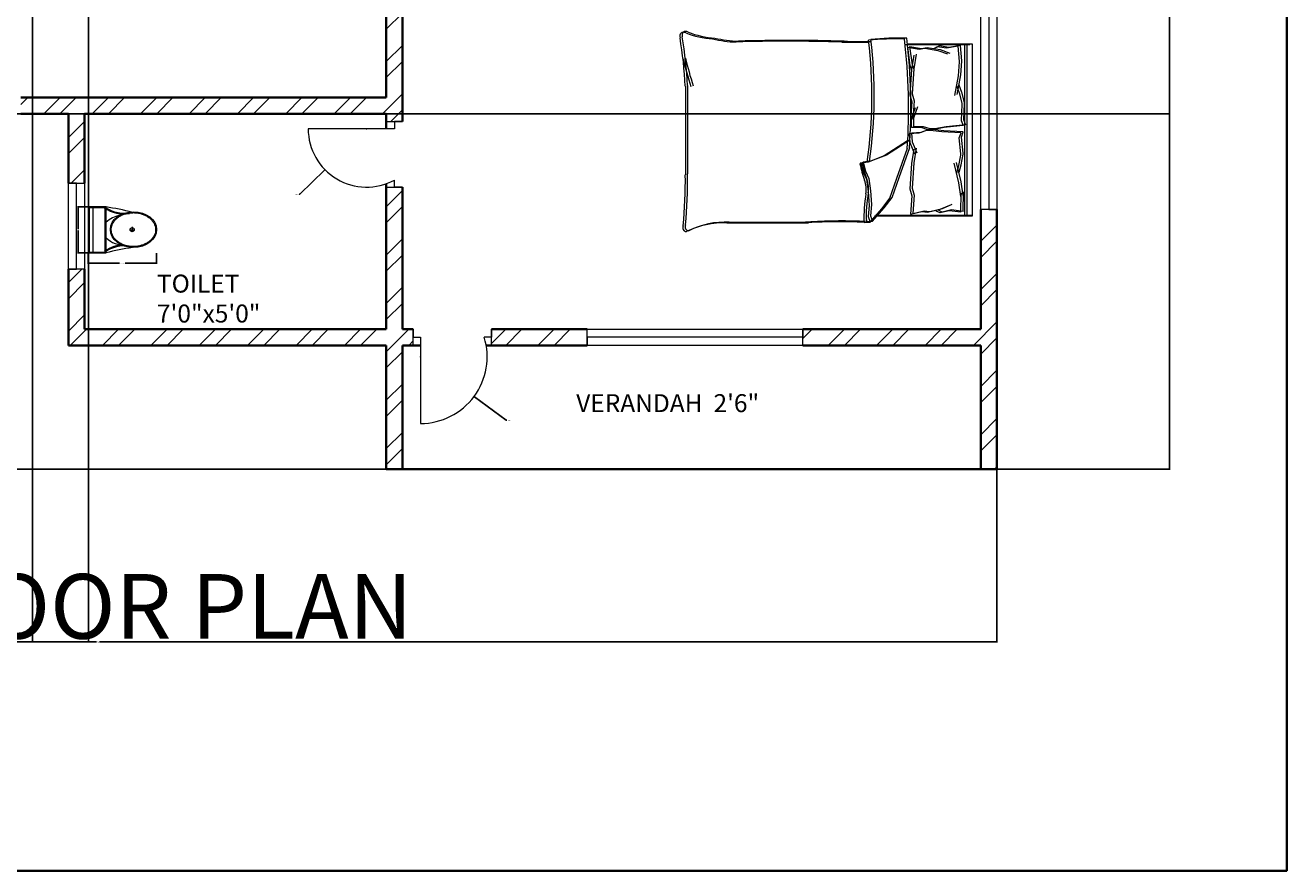
# Model space of a CAD drawing. Units: inches. Extents: x 2008 to 2657, y 1077 to 2165.
# Tile 5 of 16: x 2306 to 2657, y 1077 to 1312. Entities that reach past the tile are written whole.
import ezdxf

# ---------------------------------------------------------------- set-up
doc = ezdxf.new("R2010")
doc.units = ezdxf.units.IN
for name, color, linetype, lineweight in [('A-ANNO-DIMS', 2, 'Continuous', 18), ('A-ANNO-TITL', 7, 'Continuous', 35), ('A-ANNO-TTLB', 7, 'Continuous', 35), ('A-AREA-IDEN', 4, 'Continuous', 18), ('A-DOOR', 11, 'Continuous', 18), ('A-FLOR-FIXT', 8, 'Continuous', 18), ('A-FURN', 8, 'Continuous', 13), ('A-GLAZ', 191, 'Continuous', 18), ('A-WALL', 7, 'Continuous', 35)]:
    doc.layers.add(name, color=color, linetype=linetype, lineweight=lineweight)
doc.layers.add('A-WALL-PATT', color=30, linetype='Continuous', lineweight=13, true_color=0xf8991e)
doc.styles.get("Standard").update_dxf_attribs({"font": 'arial.ttf'})
doc.dimstyles.get("Standard").update_dxf_attribs({"dimtxt": 0.18, "dimasz": 0.18, "dimexe": 0.18, "dimexo": 0.0625, "dimgap": 0.09, "dimtad": 0, "dimtih": 1, "dimtoh": 1, "dimdec": 4, "dimzin": 0, "dimdsep": 46, "dimtxsty": 'Standard', "dimcen": 0.09, "dimadec": 0, "dimazin": 0, "dimtfac": 1, "dimtdec": 4, "dimtofl": 0, "dimtmove": 0, "dimatfit": 3, "dimfxl": 1, "dimtolj": 1, "dimtzin": 0, "dimarcsym": 0})

# ---------------------------------------------------------------- blocks, each defined once
blk = doc.blocks.new('A$C31115884')
for p, q in [((283, 498), (223, 498)), ((258, 466), (258, 523)), ((0, 200), (0, 0)), ((520, 200), (0, 200)), ((10, 190), (10, 10)), ((510, 190), (10, 190)), ((510, 10), (510, 190)), ((520, 0), (520, 200)), ((510, 54), (0, 54)), ((10, 10), (510, 10)), ((0, 0), (520, 0))]:
    blk.add_line(p, q)
blk.add_circle((256, 496), 23.6)
for centre, radius, start, end in [((2778, -205), 2807, 165.4549, 171.7133), ((-295, 403), 365, 324.2091, 9.3499), ((-295, 403), 375, 324.2091, 9.3499), ((806, 403), 365, 170.6501, 215.7909), ((3237, 905), 2807, 188.2867, 194.5451), ((384, 406), 293, 190.2774, 224.1564), ((139, 406), 293, 315.8436, 2.6563), ((806, 403), 375, 179.2036, 215.7909)]:
    blk.add_arc(centre, radius, start, end)
blk.add_ellipse((256, 510), major_axis=(0, -261), ratio=0.772727)
blk.add_open_spline([(256, 259), (263, 259), (270, 260), (288, 262), (299, 265), (320, 273), (330, 278), (350, 291), (360, 299), (378, 316), (386, 326), (402, 347), (409, 358), (421, 383), (427, 395), (436, 422), (440, 436), (445, 465), (447, 480), (448, 509), (448, 524), (445, 553), (443, 568), (436, 596), (432, 610), (422, 636), (416, 649), (402, 672), (395, 683), (379, 703), (370, 712), (351, 728), (341, 735), (321, 746), (310, 751), (289, 757), (278, 759), (256, 761), (245, 761), (223, 757), (212, 754), (191, 746), (181, 741), (161, 728), (151, 720), (133, 703), (125, 693), (110, 672), (103, 660), (90, 636), (85, 623), (76, 596), (72, 582), (67, 553), (66, 538), (64, 509), (65, 494), (68, 465), (70, 450), (77, 422), (81, 408), (91, 382), (97, 370), (111, 346), (118, 335), (135, 316), (144, 307), (162, 291), (172, 284), (193, 273), (203, 269), (225, 262), (236, 260), (250, 259), (253, 259), (256, 259)], degree=3, knots=[0, 0, 0, 0, 0.110105, 0.110105, 0.285049, 0.285049, 0.459994, 0.459994, 0.634938, 0.634938, 0.809882, 0.809882, 0.984827, 0.984827, 1.159771, 1.159771, 1.334715, 1.334715, 1.50966, 1.50966, 1.684604, 1.684604, 1.859549, 1.859549, 2.034493, 2.034493, 2.209437, 2.209437, 2.384382, 2.384382, 2.559326, 2.559326, 2.73427, 2.73427, 2.909215, 2.909215, 3.084159, 3.084159, 3.259103, 3.259103, 3.434048, 3.434048, 3.608992, 3.608992, 3.783936, 3.783936, 3.958881, 3.958881, 4.133825, 4.133825, 4.30877, 4.30877, 4.483714, 4.483714, 4.658658, 4.658658, 4.833603, 4.833603, 5.008547, 5.008547, 5.183491, 5.183491, 5.358436, 5.358436, 5.53338, 5.53338, 5.708324, 5.708324, 5.883269, 5.883269, 6.058213, 6.058213, 6.233158, 6.233158, 6.283185, 6.283185, 6.283185, 6.283185])
blk = doc.blocks.new('BED-DOUBLE')
for p, q in [((27.75, 52.87), (24.5, 49.16)), ((27.75, 52.87), (24.5, 49.16)), ((28.39, 53.1), (25.14, 49.39)), ((28.39, 53.1), (25.14, 49.39)), ((29.49, 52.95), (27.75, 52.87, 3.87)), ((29.49, 52.95), (27.75, 52.87, 3.87)), ((28.37, 51.33), (27.75, 52.87)), ((28.37, 51.33), (27.75, 52.87)), ((30.13, 53.18), (28.39, 53.1, 3.87)), ((30.13, 53.18), (28.39, 53.1, 3.87)), ((29, 51.56), (28.39, 53.1)), ((29, 51.56), (28.39, 53.1)), ((0, 51.49), (0.64, 51.49)), ((0, 3.48), (0, 51.49)), ((0, 51.27), (26.61, 51.27)), ((0, 51.27), (26.61, 51.27)), ((0.64, 51.49), (27.25, 51.49)), ((0.64, 51.49), (27.25, 51.49)), ((1.53, 3.48), (1.53, 51.27)), ((1.53, 3.48), (1.53, 51.27)), ((2.17, 3.7), (2.17, 51.49)), ((2.17, 3.7), (2.17, 51.49)), ((2.56, 50.11), (2.46, 44.71)), ((2.56, 50.11), (2.46, 44.71)), ((2.56, 50.11), (5.77, 49.73)), ((2.56, 50.11), (5.77, 49.73)), ((3.2, 50.34), (3.1, 44.94)), ((3.2, 50.34), (3.1, 44.94)), ((3.2, 50.34), (6.41, 49.96)), ((3.2, 50.34), (6.41, 49.96)), ((8.26, 49.31), (5.58, 48.13)), ((8.26, 49.31), (5.58, 48.13)), ((5.77, 49.73), (8.34, 50.33)), ((5.77, 49.73), (8.34, 50.33)), ((8.9, 49.54), (6.22, 48.36)), ((8.9, 49.54), (6.22, 48.36)), ((6.41, 49.96), (8.98, 50.56)), ((6.41, 49.96), (8.98, 50.56)), ((11.83, 50.11), (8.26, 49.31)), ((11.83, 50.11), (8.26, 49.31)), ((8.34, 50.33), (9.38, 49.82)), ((8.34, 50.33), (9.38, 49.81)), ((12.47, 50.34), (8.9, 49.54)), ((12.47, 50.34), (8.9, 49.54)), ((8.98, 50.56), (10.02, 50.04)), ((8.98, 50.56), (10.02, 50.04)), ((13.43, 49.92), (11.83, 50.11)), ((13.43, 49.92), (11.83, 50.11)), ((14.07, 50.15), (12.47, 50.34)), ((14.07, 50.15), (12.47, 50.34)), ((16.57, 50.7), (13.43, 49.92)), ((16.57, 50.7), (13.43, 49.92)), ((17.21, 50.93), (14.07, 50.15)), ((17.21, 50.93), (14.07, 50.15)), ((16.17, 45.57), (16.57, 50.7)), ((16.17, 45.57), (16.57, 50.7)), ((16.81, 45.8), (17.21, 50.93)), ((16.81, 45.8), (17.21, 50.93)), ((25.14, 49.39), (22.97, 46.45)), ((25.14, 49.39), (22.97, 46.45)), ((28.06, 48.23), (28.37, 51.33)), ((28.06, 48.23), (28.37, 51.33)), ((28.7, 48.46), (29, 51.56)), ((28.7, 48.46), (29, 51.56)), ((2.46, 44.71), (2.54, 45.71)), ((2.46, 44.71), (2.54, 45.71)), ((2.54, 45.71), (3.07, 41.91)), ((2.54, 45.71), (3.07, 41.91)), ((3.1, 44.94), (3.18, 45.94)), ((3.1, 44.94), (3.18, 45.94)), ((3.18, 45.94), (3.71, 42.14)), ((3.18, 45.94), (3.71, 42.14)), ((17.37, 43.84), (16.81, 45.8)), ((17.37, 43.83), (16.81, 45.8)), ((22.33, 46.22), (20.32, 40.64)), ((22.33, 46.22), (20.32, 40.64)), ((22.97, 46.45), (20.96, 40.87)), ((22.97, 46.45), (20.96, 40.87)), ((24.5, 49.16), (22.33, 46.22)), ((24.5, 49.16), (22.33, 46.22)), ((28.37, 44.36), (28.06, 48.23)), ((28.37, 44.36), (28.06, 48.23)), ((29, 44.59), (28.7, 48.46)), ((29, 44.59), (28.7, 48.46)), ((16.73, 43.61), (16.17, 45.57)), ((16.73, 43.61), (16.17, 45.57)), ((16.3, 36.6), (16.73, 43.61)), ((16.3, 36.6), (16.73, 43.61)), ((16.93, 36.83), (17.37, 43.84)), ((16.93, 36.82), (17.37, 43.83)), ((28.83, 40.95), (28.37, 44.36)), ((28.83, 40.95), (28.37, 44.36)), ((29.47, 41.18), (29, 44.59)), ((29.47, 41.18), (29, 44.59)), ((3.07, 41.91), (4.42, 36.5)), ((3.07, 41.91), (4.42, 36.5)), ((3.67, 39.2), (3.08, 37.14)), ((3.67, 39.2), (3.08, 37.14)), ((3.71, 42.14), (5.06, 36.72)), ((3.71, 42.14), (5.06, 36.72)), ((4.31, 39.43), (3.72, 37.36)), ((4.31, 39.43), (3.72, 37.36)), ((20.32, 40.64), (17.38, 32.31)), ((20.32, 40.64), (17.38, 32.31)), ((20.96, 40.87), (18.02, 32.54)), ((20.96, 40.87), (18.02, 32.53)), ((29.76, 38.94), (28.83, 40.95)), ((29.76, 38.94), (28.83, 40.95)), ((30.4, 39.17), (29.47, 41.18)), ((30.4, 39.17), (29.47, 41.18)), ((30.38, 36.46), (29.76, 38.94)), ((30.38, 36.46), (29.76, 38.94)), ((31.02, 36.69), (30.4, 39.17)), ((31.02, 36.69), (30.4, 39.17)), ((79.25, 15.06), (79.25, 39.68)), ((79.25, 15.06), (79.25, 39.68)), ((79.88, 15.29), (79.88, 39.91)), ((79.88, 15.29), (79.88, 39.91)), ((3.08, 37.14), (2.54, 34.21)), ((3.08, 37.14), (2.54, 34.2)), ((3.72, 37.36), (3.18, 34.43)), ((3.72, 37.36), (3.18, 34.43)), ((15.63, 32.56), (16.3, 36.6)), ((15.63, 32.56), (16.3, 36.6)), ((16.27, 32.79), (16.93, 36.83)), ((16.27, 32.79), (16.93, 36.82)), ((23.88, 34.45), (28.37, 36.15)), ((23.88, 34.45), (28.37, 36.15)), ((24.52, 34.68), (29, 36.38)), ((24.52, 34.68), (29, 36.38)), ((28.37, 36.15), (30.38, 36.46)), ((28.37, 36.15), (30.38, 36.46)), ((29, 36.38), (31.02, 36.69)), ((29, 36.38), (31.02, 36.69)), ((2.54, 34.21), (2.56, 33.88)), ((2.54, 34.2), (2.56, 33.88)), ((2.56, 33.88), (2.98, 29.46)), ((2.56, 33.88), (2.98, 29.46)), ((3.18, 34.43), (3.2, 34.11)), ((3.18, 34.43), (3.2, 34.11)), ((3.2, 34.11), (3.62, 29.68)), ((3.2, 34.11), (3.62, 29.68)), ((16.74, 30.75), (15.45, 33.82)), ((16.74, 30.75), (15.45, 33.82)), ((17.38, 30.98), (16.09, 34.05)), ((17.38, 30.98), (16.09, 34.05)), ((17.38, 30.26), (23.88, 34.45)), ((17.38, 30.26), (23.88, 34.45)), ((18.02, 30.49), (24.52, 34.68)), ((18.02, 30.49), (24.52, 34.68)), ((2.98, 29.46), (2.49, 27.98)), ((2.98, 29.46), (2.49, 27.98)), ((3.62, 29.68), (3.13, 28.21)), ((3.62, 29.68), (3.13, 28.21)), ((3.13, 28.21), (8.51, 27.96)), ((3.13, 28.21), (8.51, 27.96)), ((12.38, 27.44), (14.22, 28.13)), ((12.38, 27.44), (14.22, 28.13)), ((13.02, 27.66), (14.86, 28.36)), ((13.02, 27.66), (14.86, 28.36)), ((14.22, 28.13), (16.89, 28.3)), ((14.22, 28.13), (16.89, 28.3)), ((14.86, 28.36), (17.53, 28.53)), ((14.86, 28.36), (17.53, 28.53)), ((16.89, 28.3), (16.74, 30.75)), ((16.89, 28.3), (16.74, 30.75)), ((17.53, 28.53), (17.38, 30.98)), ((17.53, 28.53), (17.38, 30.98)), ((1.87, 25.98), (7.22, 26.56)), ((1.87, 25.98), (7.22, 26.56)), ((2.45, 24.54), (1.87, 25.98)), ((2.45, 24.54), (1.87, 25.98)), ((2.49, 27.98), (7.87, 27.73)), ((2.49, 27.98), (7.87, 27.73)), ((2.51, 26.21), (7.86, 26.79)), ((2.51, 26.21), (7.86, 26.79)), ((3.09, 24.77), (2.51, 26.21)), ((3.09, 24.77), (2.51, 26.21)), ((2.94, 20.32), (3.09, 24.77)), ((2.94, 20.32), (3.09, 24.77)), ((7.22, 26.56), (10.4, 27.14)), ((7.22, 26.56), (10.4, 27.14)), ((7.86, 26.79), (11.04, 27.37)), ((7.86, 26.79), (11.04, 27.37)), ((7.87, 27.73), (11.08, 27.36)), ((7.87, 27.73), (11.08, 27.36)), ((8.51, 27.96), (11.72, 27.58)), ((8.51, 27.96), (11.72, 27.58)), ((10.4, 27.14), (11.7, 27.14)), ((10.4, 27.14), (11.7, 27.14)), ((11.04, 27.37), (12.34, 27.37)), ((11.04, 27.37), (12.34, 27.37)), ((11.08, 27.36), (12.38, 27.44)), ((11.08, 27.36), (12.38, 27.44)), ((11.7, 27.14), (13.58, 26.56)), ((11.7, 27.14), (13.58, 26.56)), ((11.72, 27.58), (13.02, 27.66)), ((11.72, 27.58), (13.02, 27.66)), ((12.34, 27.37), (14.22, 26.79)), ((12.34, 27.37), (14.22, 26.79)), ((13.58, 26.56), (16.26, 26.56)), ((13.58, 26.56), (16.26, 26.56)), ((14.22, 26.79), (16.9, 26.79)), ((14.22, 26.79), (16.9, 26.79)), ((16.26, 26.56), (16.26, 24.1)), ((16.26, 26.56), (16.26, 24.1)), ((16.81, 19.61), (17.21, 24.74)), ((16.81, 19.61), (17.21, 24.74)), ((16.9, 26.79), (16.9, 24.33)), ((16.9, 26.79), (16.9, 24.33)), ((2.3, 20.09), (2.45, 24.54)), ((2.3, 20.09), (2.45, 24.54)), ((16.26, 24.1), (15.17, 20.96)), ((16.26, 24.1), (15.17, 20.96)), ((16.9, 24.33), (15.81, 21.19)), ((16.9, 24.33), (15.81, 21.19)), ((16.17, 19.38), (16.57, 24.52)), ((16.17, 19.38), (16.57, 24.52)), ((2.3, 19.77), (2.3, 20.09)), ((2.3, 19.77), (2.3, 20.09)), ((3.03, 16.88), (2.3, 19.77)), ((3.03, 16.88), (2.3, 19.77)), ((2.94, 20), (2.94, 20.32)), ((2.94, 20), (2.94, 20.32)), ((3.67, 17.11), (2.94, 20)), ((3.67, 17.11), (2.94, 20)), ((3.32, 12.11), (4.33, 17.6)), ((3.32, 12.11), (4.33, 17.6)), ((3.96, 12.34), (4.97, 17.83)), ((3.96, 12.34), (4.97, 17.83)), ((16.73, 17.42), (16.17, 19.38)), ((16.73, 17.42), (16.17, 19.38)), ((17.37, 17.65), (16.81, 19.61)), ((17.37, 17.65), (16.81, 19.61)), ((16.93, 10.64), (17.37, 17.65)), ((16.93, 10.64), (17.37, 17.65)), ((3.75, 14.86), (3.03, 16.88)), ((3.75, 14.86), (3.03, 16.88)), ((4.39, 15.08), (3.67, 17.11)), ((4.39, 15.08), (3.67, 17.11)), ((16.3, 10.41), (16.73, 17.42)), ((16.3, 10.41), (16.73, 17.42)), ((3.03, 8.29), (3.32, 12.11)), ((3.03, 8.29), (3.32, 12.11)), ((3.67, 8.51), (3.96, 12.34)), ((3.67, 8.51), (3.96, 12.34)), ((16.27, 6.61), (16.93, 10.64)), ((16.27, 6.61), (16.93, 10.64)), ((16.93, 10.64), (17.26, 9.51)), ((16.93, 10.64), (17.26, 9.51)), ((3.01, 8.18), (3.03, 8.29)), ((3.01, 8.18), (3.03, 8.29)), ((3.34, 3.9), (3.01, 8.18)), ((3.34, 3.9), (3.01, 8.18)), ((3.65, 8.41), (3.67, 8.51)), ((3.65, 8.41), (3.67, 8.51)), ((3.98, 4.13), (3.65, 8.41)), ((3.98, 4.13), (3.65, 8.41)), ((15.63, 6.38), (16.3, 10.41)), ((15.63, 6.38), (16.3, 10.41)), ((16.3, 10.41), (16.62, 9.28)), ((16.3, 10.41), (16.62, 9.28)), ((16.62, 9.28), (17.34, 4.18)), ((16.62, 9.28), (17.34, 4.18)), ((17.26, 9.51), (17.98, 4.41)), ((17.26, 9.51), (17.98, 4.41)), ((18.75, 3.7), (0.64, 3.7)), ((18.75, 3.7), (0.64, 3.7)), ((3.32, 3.9), (6.5, 4.47)), ((3.32, 3.89), (6.5, 4.47)), ((3.96, 4.12), (7.14, 4.7)), ((3.96, 4.12), (7.14, 4.7)), ((8.96, 5.05), (6.21, 6.06)), ((8.96, 5.05), (6.21, 6.06)), ((6.5, 4.47), (9.1, 4.04)), ((6.5, 4.47), (9.1, 4.04)), ((9.59, 5.28), (6.85, 6.29)), ((9.59, 5.28), (6.85, 6.29)), ((7.14, 4.7), (9.74, 4.27)), ((7.14, 4.7), (9.74, 4.27)), ((12.57, 4.47), (8.96, 5.05)), ((12.57, 4.47), (8.96, 5.05)), ((9.1, 4.04), (10.11, 4.62)), ((9.1, 4.04), (10.11, 4.62)), ((13.21, 4.7), (9.59, 5.28)), ((13.21, 4.7), (9.59, 5.28)), ((9.74, 4.27), (10.75, 4.85)), ((9.74, 4.27), (10.75, 4.85)), ((14.16, 4.76), (12.57, 4.47)), ((14.16, 4.76), (12.57, 4.47)), ((14.8, 4.99), (13.21, 4.7)), ((14.8, 4.99), (13.21, 4.7)), ((17.34, 4.18), (14.16, 4.76)), ((17.34, 4.18), (14.16, 4.76)), ((17.98, 4.41), (14.8, 4.99)), ((17.98, 4.41), (14.8, 4.99)), ((18.11, 3.48), (0, 3.48)), ((18.11, 3.48), (0, 3.48))]:
    blk.add_line(p, q)
for centre, radius, start, end in [((-6.66, 51.33), 36.18, 349.8763, 2.5657), ((-6.66, 51.33), 36.18, 349.8763, 2.5657), ((36.32, 182.27), 129.5, 266.9791, 273.8365), ((36.32, 182.27), 129.5, 266.9791, 273.8365), ((-6.02, 51.56), 36.18, 349.8763, 2.5657), ((-6.02, 51.56), 36.18, 349.8763, 2.5657), ((36.95, 182.49), 129.5, 266.9791, 273.8365), ((36.95, 182.49), 129.5, 266.9791, 273.8365), ((67.82, -4508.74), 4561.86, 90.00217, 90.28689), ((67.82, -4508.74), 4561.86, 90.00217, 90.28689), ((68.46, -4508.51), 4561.86, 90.00217, 90.28689), ((68.46, -4508.51), 4561.86, 90.00217, 90.28689), ((68.67, 76.16), 23.07, 267.4714, 296.4681), ((68.67, 76.16), 23.07, 267.4714, 296.4681), ((69.31, 76.39), 23.07, 267.4714, 296.4681), ((69.31, 76.39), 23.07, 267.4714, 296.4681), ((78.87, 54.41), 1.1, 332.6588, 86.02), ((78.87, 54.41), 1.1, 332.6588, 86.02), ((212.28, 41.15), 133.04, 174.4998, 180.6351), ((212.28, 41.15), 133.04, 174.4998, 180.6351), ((79.51, 54.64), 1.1, 332.6588, 86.02), ((79.51, 54.64), 1.1, 332.6588, 86.02), ((212.92, 41.38), 133.04, 174.4998, 180.6351), ((212.92, 41.38), 133.04, 174.4998, 180.6351), ((35.07, 43.74), 6.22, 168.6608, 203.7384), ((35.07, 43.74), 6.22, 168.6608, 203.7384), ((35.71, 43.97), 6.22, 168.6608, 203.7384), ((35.71, 43.97), 6.22, 168.6608, 203.7384), ((1.48, 31.15), 29.65, 10.6617, 19.8806), ((1.48, 31.15), 29.65, 10.6617, 19.8806), ((2.12, 31.38), 29.65, 10.6617, 19.8806), ((2.12, 31.38), 29.65, 10.6617, 19.8806), ((156.32, 17.76), 129.02, 171.7845, 186.9006), ((156.32, 17.76), 129.02, 171.7845, 186.9006), ((156.96, 17.98), 129.02, 171.7845, 186.9006), ((156.96, 17.98), 129.02, 171.7845, 186.9006), ((30.44, 36.64), 0.185, 250.2464, 1.1377), ((30.44, 36.64), 0.185, 250.2464, 1.1377), ((31.08, 36.87), 0.185, 250.2464, 1.1377), ((31.08, 36.86), 0.185, 250.2464, 1.1377), ((182.05, 21.36), 164.97, 176.0865, 186.7821), ((182.05, 21.36), 164.97, 176.0865, 186.7821), ((182.69, 21.59), 164.97, 176.0865, 186.7821), ((182.69, 21.59), 164.97, 176.0865, 186.7821), ((-23.71, -17.22), 106.46, 13.3832, 17.7053), ((-23.71, -17.22), 106.46, 13.3832, 17.7053), ((-23.07, -16.99), 106.46, 13.3832, 17.7053), ((-23.07, -16.99), 106.46, 13.3832, 17.7053), ((200.84, 21.43), 121.76, 182.9958, 189.4091), ((200.84, 21.43), 121.76, 182.9958, 189.4091), ((201.48, 21.66), 121.76, 182.9958, 189.4091), ((201.48, 21.66), 121.76, 182.9958, 189.4091), ((20.1, 85.16), 83.31, 268.7218, 275.604), ((20.1, 85.16), 83.31, 268.7218, 275.604), ((20.74, 85.39), 83.31, 268.7218, 275.604), ((20.74, 85.39), 83.31, 268.7218, 275.604), ((31.17, -167.31), 170.11, 88.4762, 91.0082), ((31.17, -167.31), 170.11, 88.4762, 91.0082), ((31.81, -167.08), 170.11, 88.4762, 91.0082), ((31.81, -167.08), 170.11, 88.4762, 91.0082), ((50.61, 484.82), 482.31, 268.2277, 271.7185), ((50.61, 484.82), 482.31, 268.2277, 271.7185), ((51.25, 485.05), 482.31, 268.2277, 271.7185), ((51.25, 485.05), 482.31, 268.2277, 271.7185), ((64.52, -26.9), 29.63, 76.0648, 88.9113), ((64.52, -26.9), 29.63, 76.0648, 88.9113), ((65.15, -26.67), 29.63, 76.0648, 88.9113), ((65.15, -26.67), 29.63, 76.0648, 88.9113), ((70.28, -21.66), 23.56, 67.9751, 86.652), ((70.28, -21.66), 23.56, 67.9751, 86.652), ((70.92, -21.43), 23.56, 67.9751, 86.652), ((70.92, -21.43), 23.56, 67.9751, 86.652), ((79.72, 1.09), 1.09, 236.1736, 23.4781), ((79.72, 1.09), 1.09, 236.1736, 23.4781), ((80.36, 1.32), 1.09, 236.1736, 23.4781), ((80.36, 1.32), 1.09, 236.1736, 23.4781)]:
    blk.add_arc(centre, radius, start, end)
blk = doc.blocks.new('WIN-60IN-B')
for p, q in [((0, 4.5), (0, 0)), ((0, 4.5), (60, 4.5)), ((60, 2.25), (60, 4.5)), ((60, 4.5), (60, 0)), ((0, 0), (0, 2.25)), ((0, 2.25), (60, 2.25)), ((60, 0), (0, 0))]:
    blk.add_line(p, q)
blk = doc.blocks.new('WIN-24IN-A')
for p, q in [((0, 24), (4.5, 24)), ((0, 0), (0, 24)), ((4.5, 24), (2.25, 24)), ((2.25, 24), (2.25, 0)), ((4.5, 24), (4.5, 0)), ((4.5, 0), (0, 0)), ((2.25, 0), (4.5, 0))]:
    blk.add_line(p, q)
blk = doc.blocks.new('*D13')
at = {"layer": 'A-ANNO-DIMS', "color": 0, "lineweight": -2, "transparency": 16777216}
for p, q in [((2323.8, 1248.84), (2323.8, 1245.87)), ((2342.77, 1248.84), (2342.77, 1245.87)), ((2323.98, 1246.05), (2332.51, 1246.05)), ((2342.59, 1246.05), (2334.06, 1246.05))]:
    blk.add_line(p, q, dxfattribs=at)
at = {"layer": 'A-ANNO-DIMS', "color": 0, "transparency": 16777216}
for points in [[(2323.98, 1246.08), (2323.98, 1246.02), (2323.8, 1246.05)], [(2342.59, 1246.08), (2342.59, 1246.02), (2342.77, 1246.05)]]:
    blk.add_solid(points, dxfattribs=at)
at = {"layer": 'Defpoints', "color": 0, "transparency": 16777216}
for p in [(2323.8, 1248.9), (2342.77, 1248.9), (2342.77, 1246.05)]:
    blk.add_point(p, dxfattribs=at)
at = {"layer": 'A-ANNO-DIMS', "color": 0, "transparency": 16777216, "insert": (2333.29, 1246.05), "char_height": 0.18, "attachment_point": 5}
blk.add_mtext('\\A1;WC 19 TYP.', dxfattribs=at)
blk = doc.blocks.new('*D14')
at = {"layer": 'A-ANNO-DIMS', "color": 0, "lineweight": -2, "transparency": 16777216}
for p, q in [((2323.73, 1261.71), (2320.77, 1261.71)), ((2320.95, 1261.53), (2320.95, 1255.49)), ((2320.95, 1249.08), (2320.95, 1255.12)), ((2323.73, 1248.9), (2320.77, 1248.9))]:
    blk.add_line(p, q, dxfattribs=at)
at = {"layer": 'A-ANNO-DIMS', "color": 0, "transparency": 16777216}
for points in [[(2320.92, 1261.53), (2320.98, 1261.53), (2320.95, 1261.71)], [(2320.92, 1249.08), (2320.98, 1249.08), (2320.95, 1248.9)]]:
    blk.add_solid(points, dxfattribs=at)
at = {"layer": 'Defpoints', "color": 0, "transparency": 16777216}
for p in [(2323.8, 1261.71), (2320.95, 1248.9), (2323.8, 1248.9)]:
    blk.add_point(p, dxfattribs=at)
at = {"layer": 'A-ANNO-DIMS', "color": 0, "transparency": 16777216, "insert": (2320.95, 1255.3), "char_height": 0.18, "attachment_point": 5}
blk.add_mtext('\\A1;13 TYP.', dxfattribs=at)
blk = doc.blocks.new('*D31')
at = {"layer": 'A-ANNO-DIMS', "color": 0, "lineweight": -2, "transparency": 16777216}
for p, q in [((2076.26, 1562.18), (2076.26, 1140.44)), ((2576.76, 1188.61), (2576.76, 1140.44)), ((2076.44, 1140.62), (2326.12, 1140.62)), ((2576.58, 1140.62), (2326.91, 1140.62))]:
    blk.add_line(p, q, dxfattribs=at)
at = {"layer": 'A-ANNO-DIMS', "color": 0, "transparency": 16777216}
for points in [[(2076.44, 1140.65), (2076.44, 1140.59), (2076.26, 1140.62)], [(2576.58, 1140.65), (2576.58, 1140.59), (2576.76, 1140.62)]]:
    blk.add_solid(points, dxfattribs=at)
at = {"layer": 'Defpoints', "color": 0, "transparency": 16777216}
for p in [(2076.26, 1562.24), (2576.76, 1188.67), (2576.76, 1140.62)]:
    blk.add_point(p, dxfattribs=at)
at = {"layer": 'A-ANNO-DIMS', "color": 0, "transparency": 16777216, "insert": (2326.51, 1140.62), "char_height": 0.18, "attachment_point": 5}
blk.add_mtext('\\A1;500.5', dxfattribs=at)
blk = doc.blocks.new('*D32')
at = {"layer": 'A-ANNO-DIMS', "color": 0, "lineweight": -2, "transparency": 16777216}
for p, q in [((2576.82, 2094.67), (2624.99, 2094.67)), ((2624.81, 2094.49), (2624.81, 1641.86)), ((2624.81, 1188.85), (2624.81, 1641.49)), ((2576.82, 1188.67), (2624.99, 1188.67))]:
    blk.add_line(p, q, dxfattribs=at)
at = {"layer": 'A-ANNO-DIMS', "color": 0, "transparency": 16777216}
for points in [[(2624.78, 2094.49), (2624.84, 2094.49), (2624.81, 2094.67)], [(2624.78, 1188.85), (2624.84, 1188.85), (2624.81, 1188.67)]]:
    blk.add_solid(points, dxfattribs=at)
at = {"layer": 'Defpoints', "color": 0, "transparency": 16777216}
for p in [(2576.76, 2094.67), (2624.81, 2094.67), (2576.76, 1188.67)]:
    blk.add_point(p, dxfattribs=at)
at = {"layer": 'A-ANNO-DIMS', "color": 0, "transparency": 16777216, "insert": (2624.81, 1641.67), "char_height": 0.18, "attachment_point": 5}
blk.add_mtext('\\A1;906', dxfattribs=at)
blk = doc.blocks.new('*D50')
at = {"layer": 'A-ANNO-DIMS', "color": 0, "lineweight": -2, "transparency": 16777216}
for p, q in [((2250.82, 1287.67), (2624.99, 1287.67)), ((2624.81, 1287.49), (2624.81, 1238.36)), ((2624.81, 1188.85), (2624.81, 1237.99)), ((2250.82, 1188.67), (2624.99, 1188.67))]:
    blk.add_line(p, q, dxfattribs=at)
at = {"layer": 'A-ANNO-DIMS', "color": 0, "transparency": 16777216}
for points in [[(2624.78, 1287.49), (2624.84, 1287.49), (2624.81, 1287.67)], [(2624.78, 1188.85), (2624.84, 1188.85), (2624.81, 1188.67)]]:
    blk.add_solid(points, dxfattribs=at)
at = {"layer": 'Defpoints', "color": 0, "transparency": 16777216}
for p in [(2250.76, 1287.67), (2624.81, 1287.67), (2250.76, 1188.67)]:
    blk.add_point(p, dxfattribs=at)
at = {"layer": 'A-ANNO-DIMS', "color": 0, "transparency": 16777216, "insert": (2624.81, 1238.17), "char_height": 0.18, "attachment_point": 5}
blk.add_mtext('\\A1;99', dxfattribs=at)
blk = doc.blocks.new('*D64')
at = {"layer": 'A-ANNO-DIMS', "color": 0, "lineweight": -2, "transparency": 16777216}
for p, q in [((2308.25, 1777.08), (2308.25, 1140.44)), ((2323.83, 1776.91), (2323.83, 1140.44)), ((2308.43, 1140.62), (2315.59, 1140.62)), ((2323.65, 1140.62), (2316.49, 1140.62))]:
    blk.add_line(p, q, dxfattribs=at)
at = {"layer": 'A-ANNO-DIMS', "color": 0, "transparency": 16777216}
for points in [[(2308.43, 1140.65), (2308.43, 1140.59), (2308.25, 1140.62)], [(2323.65, 1140.65), (2323.65, 1140.59), (2323.83, 1140.62)]]:
    blk.add_solid(points, dxfattribs=at)
at = {"layer": 'Defpoints', "color": 0, "transparency": 16777216}
for p in [(2308.25, 1777.15), (2323.83, 1776.97), (2323.83, 1140.62)]:
    blk.add_point(p, dxfattribs=at)
at = {"layer": 'A-ANNO-DIMS', "color": 0, "transparency": 16777216, "insert": (2316.04, 1140.62), "char_height": 0.18, "attachment_point": 5}
blk.add_mtext('\\A1;15.572', dxfattribs=at)
blk = doc.blocks.new('*D83')
at = {"layer": 'A-ANNO-DIMS', "color": 0, "lineweight": -2, "transparency": 16777216}
for p, q in [((2416.19, 1219.99), (2416.37, 1219.99)), ((2416.28, 1219.9), (2416.28, 1220.08)), ((2440.16, 1202.33), (2431.35, 1208.84)), ((2440.34, 1202.33), (2440.16, 1202.33))]:
    blk.add_line(p, q, dxfattribs=at)
at = {"layer": 'A-ANNO-DIMS', "color": 0, "transparency": 16777216}
blk.add_solid([(2431.37, 1208.87), (2431.33, 1208.82), (2431.21, 1208.95)], dxfattribs=at)
at = {"layer": 'Defpoints', "color": 0, "transparency": 16777216}
for p in [(2416.28, 1219.99), (2431.21, 1208.95)]:
    blk.add_point(p, dxfattribs=at)
at = {"layer": 'A-ANNO-DIMS', "color": 0, "transparency": 16777216, "insert": (2440.89, 1202.33), "char_height": 0.18, "attachment_point": 5}
blk.add_mtext('\\A1;R18.562', dxfattribs=at)
blk = doc.blocks.new('*D96')
at = {"layer": 'A-ANNO-DIMS', "color": 0, "lineweight": -2, "transparency": 16777216}
for p, q in [((2401.18, 1283.47), (2401.36, 1283.47)), ((2401.27, 1283.38), (2401.27, 1283.56)), ((2382.72, 1265.24), (2389.55, 1271.95)), ((2382.54, 1265.24), (2382.72, 1265.24))]:
    blk.add_line(p, q, dxfattribs=at)
at = {"layer": 'A-ANNO-DIMS', "color": 0, "transparency": 16777216}
blk.add_solid([(2389.53, 1271.97), (2389.57, 1271.93), (2389.68, 1272.08)], dxfattribs=at)
at = {"layer": 'Defpoints', "color": 0, "transparency": 16777216}
for p in [(2401.27, 1283.47), (2389.68, 1272.08)]:
    blk.add_point(p, dxfattribs=at)
at = {"layer": 'A-ANNO-DIMS', "color": 0, "transparency": 16777216, "insert": (2381.99, 1265.24), "char_height": 0.18, "attachment_point": 5}
blk.add_mtext('\\A1;R16.258', dxfattribs=at)

msp = doc.modelspace()

# ---------------------------------------------------------------- hatches: boundary and pattern name
at = {"layer": 'A-WALL-PATT'}
h = msp.add_hatch(dxfattribs=at)
h.set_pattern_fill('ANSI32', color=256)
h.paths.add_polyline_path([(2109.2619, 2094.6743), (2104.7619, 2094.6743), (2104.7619, 2072.1743), (2104.7619, 2021.6151), (2109.2619, 2021.6151), (2109.2619, 2055.6743), (2126.1387, 2055.6743), (2126.1387, 2057.9243), (2126.1387, 2060.1743), (2109.2619, 2060.1743)])
h.paths.add_polyline_path([(2223.2494, 2057.9243), (2223.2494, 2060.1743), (2186.1387, 2060.1743), (2186.1387, 2055.6743), (2223.2494, 2055.6743)])
h.paths.add_polyline_path([(2250.7619, 2072.1743), (2250.7619, 2090.1743), (2250.7619, 2094.6743), (2246.2619, 2094.6743), (2246.2619, 2060.1743), (2242.7242, 2060.1743), (2242.7242, 2055.6743), (2246.2619, 2055.6743), (2246.2619, 1899.6743), (2242.7458, 1899.6743), (2242.7458, 1897.4243), (2242.7458, 1895.1743), (2246.2619, 1895.1743), (2246.2619, 1878.8745), (2248.5119, 1878.8745), (2250.7619, 1878.8745), (2250.7619, 1991.1743), (2250.7619, 2025.6743), (2257.6798, 2025.6743), (2257.6798, 2027.9243), (2257.6798, 2030.1743), (2250.7619, 2030.1743)])
h.paths.add_polyline_path([(2411.2619, 2031.6743), (2409.0119, 2031.6743), (2406.7619, 2031.6743), (2406.7619, 2030.1743), (2322.7619, 2030.1743), (2322.7619, 2053.3443), (2318.2619, 2053.3443), (2318.2619, 2030.1743), (2305.6798, 2030.1743), (2305.6798, 2025.6743), (2318.2619, 2025.6743), (2322.7619, 2025.6743), (2406.7619, 2025.6743), (2406.7619, 1995.6743), (2406.7619, 1847.2677), (2250.7619, 1847.2677), (2250.7619, 1850.9902), (2248.5119, 1850.9902), (2246.2619, 1850.9902), (2246.2619, 1847.1743), (2246.2619, 1842.7677), (2303.0015, 1842.7677), (2303.0015, 1667.2413), (2298.4208, 1667.2413), (2298.4208, 1662.7413), (2303.0015, 1662.7413), (2303.0015, 1649.8758), (2307.5015, 1649.8758), (2307.5015, 1842.7677), (2406.7619, 1842.7677), (2411.2619, 1842.7677), (2411.2619, 1878.6743), (2415.8196, 1878.6743), (2415.8196, 1880.9243), (2415.8196, 1883.1743), (2411.2619, 1883.1743)])
h.paths.add_polyline_path([(2411.2619, 2094.6743), (2406.7619, 2094.6743), (2318.2619, 2094.6743), (2318.2619, 2077.3443), (2322.7619, 2077.3443), (2322.7619, 2090.1743), (2406.7619, 2090.1743), (2406.7619, 2072.1743), (2406.7619, 2067.6743), (2406.7619, 2052.7524), (2411.2619, 2052.7524), (2411.2619, 2055.6743), (2414.9888, 2055.6743), (2414.9888, 2057.9243), (2414.9888, 2060.1743), (2411.2619, 2060.1743), (2411.2619, 2072.1743)])
h.paths.add_polyline_path([(2576.7619, 2072.1743), (2576.7619, 2094.6743), (2572.2619, 2094.6743), (2572.2619, 2060.1743), (2525.8113, 2060.1743), (2525.8113, 2055.6743), (2572.2619, 2055.6743), (2572.2619, 1994.289), (2576.7619, 1994.289)])
h.paths.add_polyline_path([(2465.8113, 2060.1743), (2436.2802, 2060.1743), (2436.2802, 2055.6743), (2465.8113, 2055.6743), (2465.8113, 2057.9243)])
h.paths.add_polyline_path([(2576.7619, 1934.289), (2574.5119, 1934.289), (2572.2619, 1934.289), (2572.2619, 1883.1743), (2447.7027, 1883.1743), (2447.7027, 1878.6743), (2459.7619, 1878.6743), (2459.7619, 1830.4982), (2464.2619, 1830.4982), (2464.2619, 1878.6743), (2572.2619, 1878.6743), (2572.2619, 1868.4883), (2576.7619, 1868.4883)])
h.paths.add_polyline_path([(2576.7619, 1832.4883), (2572.2619, 1832.4883), (2572.2619, 1806.6743), (2464.2619, 1806.6743), (2464.2619, 1809.6629), (2459.7619, 1809.6629), (2459.7619, 1802.1743), (2483.7619, 1802.1743), (2483.7619, 1778.1743), (2488.2619, 1778.1743), (2488.2619, 1802.1743), (2572.2619, 1802.1743), (2572.2619, 1793.6101), (2576.7619, 1793.6101)])
h.paths.add_polyline_path([(2576.7619, 1769.6101), (2572.2619, 1769.6101), (2572.2619, 1754.1743), (2488.2619, 1754.1743), (2488.2619, 1757.2675), (2486.0119, 1757.2675), (2483.7619, 1757.2675), (2483.7619, 1754.1743), (2447.4528, 1754.1743), (2447.4528, 1749.6743), (2483.7619, 1749.6743), (2572.2619, 1749.6743), (2572.2619, 1715.1837), (2576.7619, 1715.1837)])
h.paths.add_polyline_path([(2576.7619, 1655.1837), (2572.2619, 1655.1837), (2572.2619, 1617.6743), (2411.2619, 1617.6743), (2411.2619, 1749.6743), (2414.2827, 1749.6743), (2414.2827, 1754.1743), (2406.7619, 1754.1743), (2406.7619, 1749.6743), (2406.7619, 1617.6743), (2307.5015, 1617.6743), (2307.5015, 1621.0007), (2305.2515, 1621.0007), (2303.0015, 1621.0007), (2303.0015, 1609.6944), (2307.5015, 1609.6944), (2307.5015, 1613.1743), (2406.7619, 1613.1743), (2406.7619, 1476.6743), (2415.532, 1476.6743), (2415.532, 1478.9243), (2415.532, 1481.1743), (2411.2619, 1481.1743), (2411.2619, 1613.1743), (2572.2619, 1613.1743), (2572.2619, 1584.6086), (2576.7619, 1584.6086)])
h.paths.add_polyline_path([(2576.7619, 1524.6086), (2572.2619, 1524.6086), (2572.2619, 1481.1743), (2483.7619, 1481.1743), (2447.5119, 1481.1743), (2447.5119, 1476.6743), (2483.7619, 1476.6743), (2483.7619, 1473.5051), (2488.2619, 1473.5051), (2488.2619, 1476.6743), (2572.2619, 1476.6743), (2572.2619, 1469.5488), (2576.7619, 1469.5488)])
h.paths.add_polyline_path([(2576.7619, 1445.5488), (2572.2619, 1445.5488), (2572.2619, 1428.6743), (2488.2619, 1428.6743), (2488.2619, 1455.6743), (2486.0119, 1455.6743), (2483.7619, 1455.6743), (2483.7619, 1428.6743), (2459.7619, 1428.6743), (2459.7619, 1422.1519), (2464.2619, 1422.1519), (2464.2619, 1424.1743), (2572.2619, 1424.1743), (2572.2619, 1407.5685), (2576.7619, 1407.5685)])
h.paths.add_polyline_path([(2576.7619, 1371.5685), (2572.2619, 1371.5685), (2572.2619, 1352.1743), (2464.2619, 1352.1743), (2464.2619, 1403.1384), (2462.0119, 1403.1384), (2459.7619, 1403.1384), (2459.7619, 1352.1743), (2446.3194, 1352.1743), (2446.3194, 1347.6743), (2572.2619, 1347.6743), (2572.2619, 1321.0291), (2576.7619, 1321.0291)])
h.paths.add_polyline_path([(2462.703, 1227.6743), (2436.0298, 1227.6743), (2436.0298, 1225.4243), (2436.0298, 1223.1743), (2462.703, 1223.1743), (2462.703, 1225.4243)])
h.paths.add_polyline_path([(2576.7619, 1261.0291), (2574.5119, 1261.0291), (2572.2619, 1261.0291), (2572.2619, 1227.6743), (2522.703, 1227.6743), (2522.703, 1223.1743), (2572.2619, 1223.1743), (2572.2619, 1188.6743), (2576.7619, 1188.6743), (2576.7619, 1193.1743), (2576.7619, 1223.1743)])
h.paths.add_polyline_path([(2414.2823, 1227.6743), (2411.2619, 1227.6743), (2411.2619, 1267.1779), (2409.0119, 1267.1779), (2406.7619, 1267.1779), (2406.7619, 1227.6743), (2322.7619, 1227.6743), (2322.7619, 1244.3623), (2318.2619, 1244.3623), (2318.2619, 1223.1743), (2406.7619, 1223.1743), (2406.7619, 1193.1743), (2406.7619, 1188.6743), (2411.2619, 1188.6743), (2411.2619, 1193.1743), (2411.2619, 1223.1743), (2414.2823, 1223.1743)])
h.paths.add_polyline_path([(2411.2619, 1347.6743), (2414.702, 1347.6743), (2414.702, 1349.9243), (2414.702, 1352.1743), (2411.2619, 1352.1743), (2411.2619, 1416.7413), (2307.5015, 1416.7413), (2307.5015, 1579.8489), (2305.2515, 1579.8489), (2303.0015, 1579.8489), (2303.0015, 1566.7413), (2299.2719, 1566.7413), (2299.2719, 1562.2413), (2303.0015, 1562.2413), (2303.0015, 1416.7413), (2246.2619, 1416.7413), (2246.2619, 1409.8616), (2250.7619, 1409.8616), (2250.7619, 1412.2413), (2406.7619, 1412.2413), (2406.7619, 1292.1743), (2304.9703, 1292.1743), (2304.9703, 1287.6743), (2318.2619, 1287.6743), (2318.2619, 1268.3623), (2322.7619, 1268.3623), (2322.7619, 1287.6743), (2406.7619, 1287.6743), (2406.7619, 1285.4748), (2411.2619, 1285.4748)])
h.paths.add_polyline_path([(2109.2619, 1262.7482), (2104.7619, 1262.7482), (2104.7619, 1223.1743), (2104.7619, 1193.1743), (2104.7619, 1188.6743), (2109.2619, 1188.6743), (2109.2619, 1223.1743), (2126.7928, 1223.1743), (2126.7928, 1225.4243), (2126.7928, 1227.6743), (2109.2619, 1227.6743)])
h.paths.add_polyline_path([(2222.3268, 1227.6743), (2186.7928, 1227.6743), (2186.7928, 1223.1743), (2222.3268, 1223.1743)])
h.paths.add_polyline_path([(2250.7619, 1287.6743), (2256.9703, 1287.6743), (2256.9703, 1289.9243), (2256.9703, 1292.1743), (2250.7619, 1292.1743), (2250.7619, 1382.2078), (2248.5119, 1382.2078), (2246.2619, 1382.2078), (2246.2619, 1347.6743), (2246.2619, 1227.6743), (2242.6068, 1227.6743), (2242.6068, 1223.1743), (2246.2619, 1223.1743), (2246.2619, 1188.6743), (2250.7619, 1188.6743), (2250.7619, 1193.1743), (2250.7619, 1227.6743)])
h.paths.add_polyline_path([(2133.2619, 1349.9243), (2133.2619, 1352.1743), (2109.2619, 1352.1743), (2109.2619, 1375.2826), (2104.7619, 1375.2826), (2104.7619, 1322.7482), (2109.2619, 1322.7482), (2109.2619, 1347.6743), (2133.2619, 1347.6743)])
h.paths.add_polyline_path([(2210.2105, 1352.1743), (2161.7619, 1352.1743), (2161.7619, 1412.2413), (2185.7619, 1412.2413), (2185.7619, 1420.1851), (2183.5119, 1420.1851), (2181.2619, 1420.1851), (2181.2619, 1416.7413), (2109.2619, 1416.7413), (2109.2619, 1452.4006), (2104.7619, 1452.4006), (2104.7619, 1399.2826), (2109.2619, 1399.2826), (2109.2619, 1412.2413), (2157.2619, 1412.2413), (2157.2619, 1352.1743), (2154.3383, 1352.1743), (2154.3383, 1347.6743), (2210.2105, 1347.6743)])
h.paths.add_polyline_path([(2185.7619, 1514.2413), (2161.7619, 1514.2413), (2161.7619, 1518.1307), (2159.5119, 1518.1307), (2157.2619, 1518.1307), (2157.2619, 1514.2413), (2109.2619, 1514.2413), (2109.2619, 1528.997), (2107.0119, 1528.997), (2104.7619, 1528.997), (2104.7619, 1488.4006), (2109.2619, 1488.4006), (2109.2619, 1509.7413), (2181.2619, 1509.7413), (2181.2619, 1441.2042), (2185.7619, 1441.2042)])
h.paths.add_polyline_path([(2270.4025, 1566.7413), (2109.2619, 1566.7413), (2080.7619, 1566.7413), (2080.7619, 1586.5643), (2076.2619, 1586.5643), (2076.2619, 1562.2413), (2080.7619, 1562.2413), (2104.7619, 1562.2413), (2104.7619, 1552.997), (2109.2619, 1552.997), (2109.2619, 1562.2413), (2157.2619, 1562.2413), (2157.2619, 1538.2413), (2161.7619, 1538.2413), (2161.7619, 1562.2413), (2205.2619, 1562.2413), (2270.4025, 1562.2413)])
h.paths.add_polyline_path([(2131.6813, 1897.4243), (2131.6813, 1899.6743), (2109.2619, 1899.6743), (2109.2619, 1961.6151), (2104.7619, 1961.6151), (2104.7619, 1886.8042), (2109.2619, 1886.8042), (2109.2619, 1895.1743), (2131.6813, 1895.1743)])
h.paths.add_polyline_path([(2185.7619, 1847.1743), (2161.7619, 1847.1743), (2161.7619, 1895.1743), (2185.7619, 1895.1743), (2211.543, 1895.1743), (2211.543, 1897.4243), (2211.543, 1899.6743), (2154.0916, 1899.6743), (2154.0916, 1897.4243), (2154.0916, 1895.1743), (2157.2619, 1895.1743), (2157.2619, 1847.1743), (2109.2619, 1847.1743), (2109.2619, 1862.8042), (2104.7619, 1862.8042), (2104.7619, 1821.243), (2109.2619, 1821.243), (2109.2619, 1842.6743), (2181.2619, 1842.6743), (2181.2619, 1840.6763), (2185.7619, 1840.6763)])
h.paths.add_polyline_path([(2109.2619, 1785.243), (2104.7619, 1785.243), (2104.7619, 1715.4691), (2109.2619, 1715.4691), (2109.2619, 1730.8423), (2157.2619, 1730.8423), (2157.2619, 1727.6404), (2161.7619, 1727.6404), (2161.7619, 1730.8423), (2185.7619, 1730.8423), (2185.7619, 1822.1438), (2183.5119, 1822.1438), (2181.2619, 1822.1438), (2181.2619, 1735.3423), (2109.2619, 1735.3423)])
h.paths.add_polyline_path([(2109.2619, 1691.4691), (2104.7619, 1691.4691), (2104.7619, 1667.2413), (2076.2619, 1667.2413), (2076.2619, 1646.5643), (2080.7619, 1646.5643), (2080.7619, 1662.7413), (2109.2619, 1662.7413), (2271.4941, 1662.7413), (2271.4941, 1664.9913), (2271.4941, 1667.2413), (2181.2619, 1667.2413), (2161.7619, 1667.2413), (2161.7619, 1708.3752), (2159.5119, 1708.3752), (2157.2619, 1708.3752), (2157.2619, 1667.2413), (2109.2619, 1667.2413)])
h.paths.add_polyline_path([(2233.1467, 1747.4973), (2270.0737, 1747.4973), (2270.0737, 1766.1547), (2233.1467, 1766.1547)], flags=9)

# ---------------------------------------------------------------- linework, layer by layer
at = {"layer": 'A-ANNO-TTLB'}
msp.add_lwpolyline([(2008.4537, 2164.5615), (2657.4477, 2164.5615), (2657.4477, 1076.8888), (2008.4537, 1076.8888)], close=True, dxfattribs=at)
at = {"layer": 'A-DOOR'}
for p, q in [((2406.7619, 1285.4748), (2411.2619, 1285.4748)), ((2411.2619, 1285.4748), (2409.0119, 1285.4748)), ((2409.0119, 1285.4748), (2409.0119, 1283.4748)), ((2409.0119, 1283.4748), (2385.0119, 1283.4748)), ((2409.0119, 1267.1779), (2409.0119, 1269.1779)), ((2406.7619, 1267.1779), (2411.2619, 1267.1779)), ((2411.2619, 1267.1779), (2409.0119, 1267.1779)), ((2414.2823, 1223.1743), (2414.2823, 1227.6743)), ((2414.2823, 1227.6743), (2414.2823, 1225.4243)), ((2436.0298, 1223.1743), (2436.0298, 1227.6743)), ((2436.0298, 1227.6743), (2436.0298, 1225.4243)), ((2414.2823, 1225.4243), (2416.2823, 1225.4243)), ((2416.2823, 1225.4243), (2416.2823, 1201.4243)), ((2436.0298, 1225.4243), (2434.0298, 1225.4243))]:
    msp.add_line(p, q, dxfattribs=at)
for centre, radius, start, end in [((2401.2702, 1283.4748), 16.2583, 180, 298.435391), ((2416.2823, 1219.9863), 18.5619, 270, 17.035772)]:
    msp.add_arc(centre, radius, start, end, dxfattribs=at)
at = {"layer": 'A-WALL'}
for p, q in [((2406.7619, 1412.2413), (2406.7619, 1292.1743)), ((2411.2619, 1347.6743), (2411.2619, 1285.4748)), ((2406.7619, 1292.1743), (2304.9703, 1292.1743)), ((2322.7619, 1292.1743), (2318.2619, 1292.1743)), ((2304.9703, 1287.6743), (2318.2619, 1287.6743)), ((2318.2619, 1287.6743), (2318.2619, 1268.3623)), ((2322.7619, 1287.6743), (2406.7619, 1287.6743)), ((2322.7619, 1268.3623), (2322.7619, 1287.6743)), ((2406.7619, 1287.6743), (2406.7619, 1283.4748)), ((2406.7619, 1268.172), (2406.7619, 1227.6743)), ((2411.2619, 1267.1779), (2411.2619, 1227.6743)), ((2572.2619, 1261.0291), (2572.2619, 1227.6743)), ((2576.7619, 1261.0291), (2576.7619, 1223.1743)), ((2318.2619, 1244.3623), (2318.2619, 1223.1743)), ((2322.7619, 1227.6743), (2322.7619, 1244.3623)), ((2406.7619, 1227.6743), (2322.7619, 1227.6743)), ((2322.7619, 1227.6743), (2406.7619, 1227.6743)), ((2411.2619, 1227.6743), (2414.2823, 1227.6743)), ((2436.0298, 1227.6743), (2462.703, 1227.6743)), ((2522.703, 1227.6743), (2572.2619, 1227.6743)), ((2318.2619, 1223.1743), (2406.7619, 1223.1743)), ((2406.7619, 1223.1743), (2406.7619, 1193.1743)), ((2411.2619, 1193.1743), (2411.2619, 1223.1743)), ((2411.2619, 1223.1743), (2416.2823, 1223.1743)), ((2434.5684, 1223.1743), (2462.703, 1223.1743)), ((2522.703, 1223.1743), (2572.2619, 1223.1743)), ((2572.2619, 1223.1743), (2572.2619, 1188.6743)), ((2576.7619, 1223.1743), (2576.7619, 1193.1743)), ((2406.7619, 1193.1743), (2406.7619, 1188.6743)), ((2411.2619, 1193.1743), (2411.2619, 1188.6743)), ((2576.7619, 1188.6743), (2576.7619, 1193.1743)), ((2406.7619, 1188.6743), (2576.7619, 1188.6743))]:
    msp.add_line(p, q, dxfattribs=at)

# ---------------------------------------------------------------- block references
at = {"layer": 'A-FLOR-FIXT', "xscale": 0.0246256636748975, "yscale": 0.0246256636748975, "zscale": 0.0246256636748975, "rotation": 270}
msp.add_blockref('A$C31115884', (2323.7975, 1261.7059), dxfattribs=at)
at = {"layer": 'A-FURN', "rotation": 180}
msp.add_blockref('BED-DOUBLE', (2569.8899, 1310.5887), dxfattribs=at)
at = {"layer": 'A-GLAZ'}
for name, p, rotation in [('WIN-60IN-B', (2572.2616, 1321.0288), 269.9999999999992), ('WIN-24IN-A', (2322.7618, 1268.3624), 180), ('WIN-60IN-B', (2522.7027, 1227.6747), 180)]:
    msp.add_blockref(name, p, dxfattribs=dict(at, rotation=rotation))

# ---------------------------------------------------------------- texts
at = {"layer": 'A-ANNO-TITL', "insert": (2196.855, 1159.5061), "char_height": 18, "attachment_point": 1}
msp.add_mtext_dynamic_manual_height_columns('FIRST FLOOR PLAN ', width=396.979192, gutter_width=12.5, heights=[0], dxfattribs=at)
at = {"layer": 'A-AREA-IDEN', "char_height": 5, "attachment_point": 1}
for s, width, insert in [('TOILET\\P7\'0"x5\'0"', 128.750892, (2342.9109, 1242.8653)), ('VERANDAH  2\'6"', 172.93008, (2459.6398, 1209.5799))]:
    msp.add_mtext_dynamic_manual_height_columns(s, width=width, gutter_width=12.5, heights=[0], dxfattribs=dict(at, insert=insert))

# ---------------------------------------------------------------- dimensions: what is measured, and where the dimension line sits
at = {"layer": 'A-ANNO-DIMS'}
for base, p1, p2, picture, middle in [((2624.8119, 2094.6743), (2576.7619, 1188.6743), (2576.7619, 2094.6743), '*D32', (2624.8119, 1641.6743)), ((2624.8119, 1287.6743), (2250.7619, 1188.6743), (2250.7619, 1287.6743), '*D50', (2624.8119, 1238.1743))]:
    dim = msp.add_linear_dim(base=base, p1=p1, p2=p2, angle=90, dimstyle='Standard', override={"dimdec": 0, "dimlfac": 1, "dimrnd": 0, "dimzin": 0, "dimdsep": 46, "dimlunit": 2}, dxfattribs=at)
    dim.commit()
    dim.dimension.update_dxf_attribs({"geometry": picture, "text_midpoint": middle})
for base, p1, p2, override, picture, middle in [((2323.8256, 1140.6243), (2308.2533, 1777.1466), (2323.8256, 1776.9735), {"dimdec": 3, "dimlfac": 1, "dimrnd": 0, "dimzin": 0, "dimdsep": 46, "dimlunit": 2}, '*D64', (2316.0395, 1140.6243)), ((2576.7619, 1140.6243), (2076.2619, 1562.2413), (2576.7619, 1188.6743), {"dimdec": 1, "dimlfac": 1, "dimrnd": 0, "dimzin": 0, "dimdsep": 46, "dimlunit": 2}, '*D31', (2326.5119, 1140.6243))]:
    dim = msp.add_linear_dim(base=base, p1=p1, p2=p2, dimstyle='Standard', override=override, dxfattribs=at)
    dim.commit()
    dim.dimension.update_dxf_attribs({"geometry": picture, "text_midpoint": middle})
for center, mpoint, picture, middle in [((2401.2702, 1283.4748), (2389.6767, 1272.0764), '*D96', (2381.9906, 1265.2374)), ((2416.2823, 1219.9863), (2431.207, 1208.95), '*D83', (2440.8906, 1202.3283))]:
    dim = msp.add_radius_dim(center=center, mpoint=mpoint, dimstyle='Standard', override={"dimdec": 3, "dimlfac": 1, "dimrnd": 0, "dimzin": 0, "dimdsep": 46, "dimlunit": 2}, dxfattribs=at)
    dim.commit()
    dim.dimension.update_dxf_attribs({"geometry": picture, "text_midpoint": middle, "dimtype": 164})
dim = msp.add_linear_dim(base=(2320.9511, 1248.9006), p1=(2323.7975, 1261.7059), p2=(2323.7975, 1248.9006), angle=270, text='<> TYP.', dimstyle='Standard', override={"dimdec": 0, "dimlfac": 1, "dimrnd": 0, "dimzin": 0, "dimdsep": 46, "dimlunit": 2}, dxfattribs=at)
dim.commit()
dim.dimension.update_dxf_attribs({"geometry": '*D14', "text_midpoint": (2320.9511, 1255.3032)})
dim = msp.add_linear_dim(base=(2342.7733, 1246.0542), p1=(2323.7975, 1248.9006), p2=(2342.7733, 1248.9006), text='WC <> TYP.', dimstyle='Standard', override={"dimdec": 0, "dimlfac": 1, "dimrnd": 0, "dimzin": 0, "dimdsep": 46, "dimlunit": 2}, dxfattribs=at)
dim.commit()
dim.dimension.update_dxf_attribs({"geometry": '*D13', "text_midpoint": (2333.2854, 1246.0542)})

doc.saveas('drawing.dxf')
